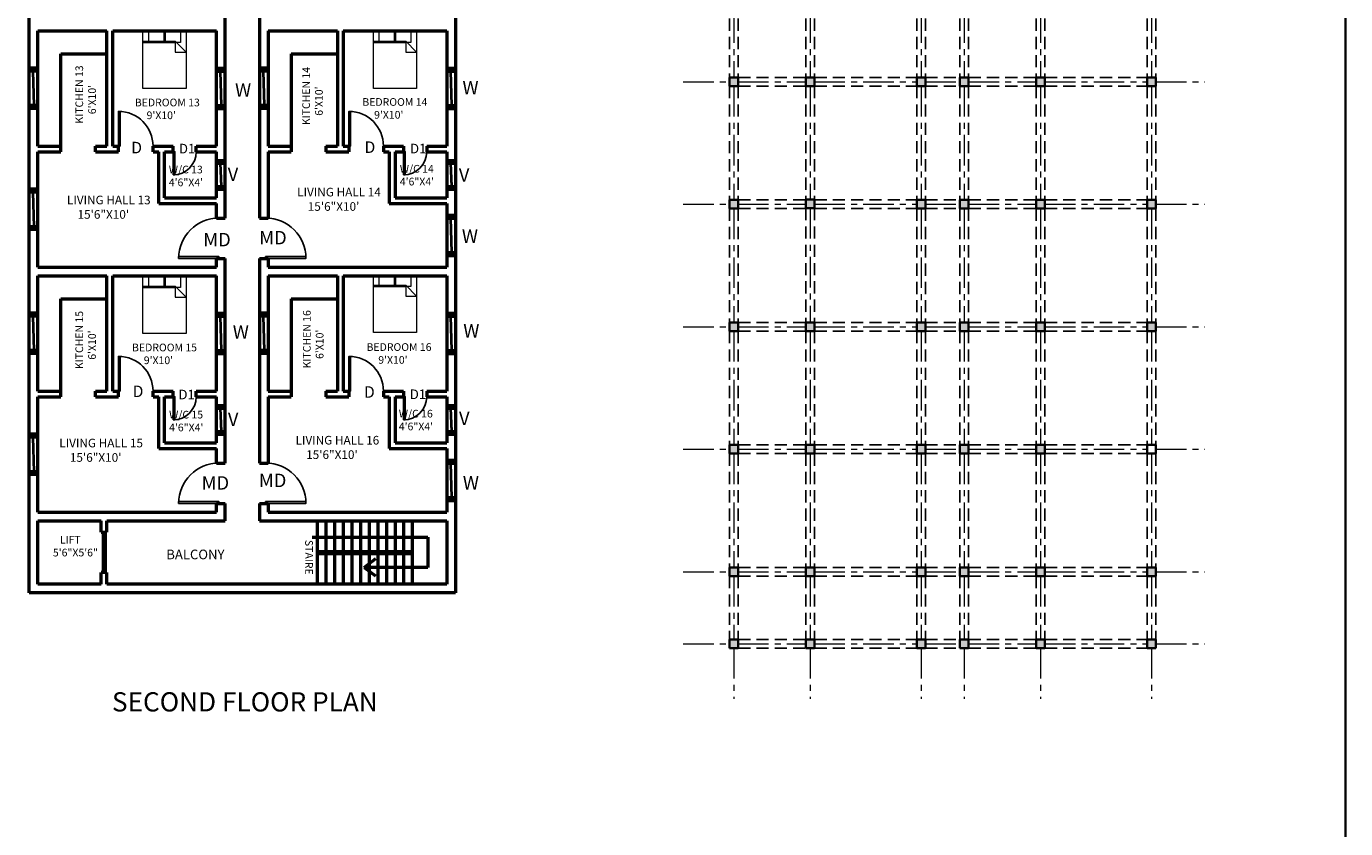
# Model space of a CAD drawing. Units: inches. Extents: x 9239 to 26065, y 6728 to 14611.
# Tile 11 of 12: x 24691 to 26065, y 13102 to 13937. Entities that reach past the tile are written whole.
import ezdxf

# ---------------------------------------------------------------- set-up
doc = ezdxf.new("R2010")
doc.units = ezdxf.units.IN
doc.header["$MEASUREMENT"] = 0
doc.linetypes.add('CENTER', pattern=[50.8, 31.75, -6.35, 6.35, -6.35])
doc.linetypes.add('DASHED', pattern=[19.05, 12.7, -6.35])
for name, color, linetype, lineweight in [('A-ANNO-TEXT', 7, 'Continuous', 18), ('A-ANNO-TTLB', 7, 'Continuous', 35), ('A-AREA-IDEN', 7, 'Continuous', 18), ('A-DOOR', 4, 'Continuous', 25), ('A-FURN', 8, 'Continuous', 18), ('A-GLAZ', 4, 'Continuous', 25), ('A-GRID', 3, 'CENTER', 18), ('A-WALL', 7, 'Continuous', 50), ('S-BEAM', 4, 'DASHED', 25), ('S-COLS', 1, 'Continuous', 35), ('S-PATT', 252, 'Continuous', 13)]:
    doc.layers.add(name, color=color, linetype=linetype, lineweight=lineweight)
doc.styles.get("Standard").update_dxf_attribs({"font": 'arial.ttf'})

# ---------------------------------------------------------------- blocks, each defined once
blk = doc.blocks.new('*U10')
for p, q in [((0, 0), (0, -6)), ((36, 0), (36, -6))]:
    blk.add_line(p, q)
blk.add_lwpolyline([(0, 0), (0, 36), (1.75, 36), (1.75, 0)], close=True)
blk.add_arc((0, 0), 36, 0, 90)
blk = doc.blocks.new('*U34')
for p, q in [((0, 0), (0, 6)), ((24, 0), (24, 6))]:
    blk.add_line(p, q)
blk.add_lwpolyline([(0, 0), (0, -24), (1.75, -24), (1.75, 0)], close=True)
blk.add_arc((0, 0), 24, 270, 0)
blk = doc.blocks.new('*U33')
for p, q in [((-40, 0), (-40, 6)), ((0, 0), (0, 6))]:
    blk.add_line(p, q)
blk.add_lwpolyline([(0, 0), (0, -40), (-1.75, -40), (-1.75, 0)], close=True)
blk.add_arc((0, 0), 40, 180, 270)
blk = doc.blocks.new('*U35')
for p, q in [((0, 0), (0, -6)), ((-40, 0), (-40, -6))]:
    blk.add_line(p, q)
blk.add_lwpolyline([(0, 0), (0, 40), (-1.75, 40), (-1.75, 0)], close=True)
blk.add_arc((0, 0), 40, 90, 180)
blk = doc.blocks.new('Bed - Queen')
for p, q in [((0, -80.00003), (0, 0)), ((0, 0), (59.99999, 0)), ((59.99999, 0), (59.99999, -80.00003)), ((0, -14.4), (44.8, -14.4)), ((44.8, -16.8), (0, -16.8)), ((7.99999, -1.2), (28.79998, -1.2)), ((7.99999, -14.4), (7.99999, -1.2)), ((28.79998, -1.2), (28.79998, -14.4)), ((31.19999, -1.2), (51.99999, -1.2)), ((31.19999, -14.4), (31.19999, -1.2)), ((59.99999, -29.6), (44.8, -14.4)), ((44.8, -14.4), (44.8, -29.6)), ((51.99999, -16.4), (46.79936, -16.4)), ((51.99999, -1.2), (51.99999, -16.4)), ((44.8, -29.6), (59.99999, -29.6)), ((59.99999, -80.00003), (0, -80.00003))]:
    blk.add_line(p, q)
blk = doc.blocks.new('WIN-36')
for p, q in [((0, 1), (36, 1)), ((0, 0.5), (36, 0.5)), ((0, 0), (36, 0))]:
    blk.add_line(p, q)
blk = doc.blocks.new('WIN-24')
for p, q in [((0, 1), (24, 1)), ((0, 0.5), (24, 0.5)), ((0, 0), (24, 0))]:
    blk.add_line(p, q)

msp = doc.modelspace()

# ---------------------------------------------------------------- hatches: boundary and pattern name
at = {"layer": 'S-PATT'}
h = msp.add_hatch(color=256, dxfattribs=at)
h.dxf.hatch_style = 1
h.paths.add_polyline_path([(25432.02, 14384.38), (25432.02, 14393.38), (25423.02, 14393.38), (25423.02, 14384.38)])
h.paths.add_polyline_path([(25511.52, 14384.38), (25511.52, 14393.38), (25502.52, 14393.38), (25502.52, 14384.38)])
h.paths.add_polyline_path([(25627.02, 14384.38), (25627.02, 14393.38), (25618.02, 14393.38), (25618.02, 14384.38)])
h.paths.add_polyline_path([(25672.02, 14393.38), (25663.02, 14393.38), (25663.02, 14384.38), (25672.02, 14384.38)])
h.paths.add_polyline_path([(25742.52, 14384.38), (25751.52, 14384.38), (25751.52, 14393.38), (25742.52, 14393.38)])
h.paths.add_polyline_path([(25858.02, 14384.38), (25867.02, 14384.38), (25867.02, 14393.38), (25858.02, 14393.38)])
h.paths.add_polyline_path([(25423.02, 14256.88), (25432.02, 14256.88), (25432.02, 14265.88), (25423.02, 14265.88)])
h.paths.add_polyline_path([(25502.52, 14256.88), (25511.52, 14256.88), (25511.52, 14265.88), (25502.52, 14265.88)])
h.paths.add_polyline_path([(25618.02, 14256.88), (25627.02, 14256.88), (25627.02, 14265.88), (25618.02, 14265.88)])
h.paths.add_polyline_path([(25672.02, 14265.88), (25663.02, 14265.88), (25663.02, 14256.88), (25672.02, 14256.88)])
h.paths.add_polyline_path([(25751.52, 14256.88), (25751.52, 14265.88), (25742.52, 14265.88), (25742.52, 14256.88)])
h.paths.add_polyline_path([(25858.02, 14256.88), (25867.02, 14256.88), (25867.02, 14265.88), (25858.02, 14265.88)])
h.paths.add_polyline_path([(25423.02, 14129.38), (25432.02, 14129.38), (25432.02, 14138.38), (25423.02, 14138.38)])
h.paths.add_polyline_path([(25511.52, 14129.38), (25511.52, 14138.38), (25502.52, 14138.38), (25502.52, 14129.38)])
h.paths.add_polyline_path([(25618.02, 14129.38), (25627.02, 14129.38), (25627.02, 14138.38), (25618.02, 14138.38)])
h.paths.add_polyline_path([(25672.02, 14138.38), (25663.02, 14138.38), (25663.02, 14129.38), (25672.02, 14129.38)])
h.paths.add_polyline_path([(25742.52, 14129.38), (25751.52, 14129.38), (25751.52, 14138.38), (25742.52, 14138.38)])
h.paths.add_polyline_path([(25867.02, 14129.38), (25867.02, 14138.38), (25858.02, 14138.38), (25858.02, 14129.38)])
h.paths.add_polyline_path([(25432.02, 14010.88), (25423.02, 14010.88), (25423.02, 14001.88), (25432.02, 14001.88)])
h.paths.add_polyline_path([(25502.52, 14010.88), (25502.52, 14001.88), (25511.52, 14001.88), (25511.52, 14010.88)])
h.paths.add_polyline_path([(25618.02, 14001.88), (25627.02, 14001.88), (25627.02, 14010.88), (25618.02, 14010.88)])
h.paths.add_polyline_path([(25672.02, 14001.88), (25672.02, 14010.88), (25663.02, 14010.88), (25663.02, 14001.88)])
h.paths.add_polyline_path([(25751.52, 14010.88), (25742.52, 14010.88), (25742.52, 14001.88), (25751.52, 14001.88)])
h.paths.add_polyline_path([(25867.02, 14010.88), (25858.02, 14010.88), (25858.02, 14001.88), (25867.02, 14001.88)])
h.paths.add_polyline_path([(25432.02, 13874.38), (25432.02, 13883.38), (25423.02, 13883.38), (25423.02, 13874.38)])
h.paths.add_polyline_path([(25502.52, 13874.38), (25511.52, 13874.38), (25511.52, 13883.38), (25502.52, 13883.38)])
h.paths.add_polyline_path([(25627.02, 13883.38), (25618.02, 13883.38), (25618.02, 13874.38), (25627.02, 13874.38)])
h.paths.add_polyline_path([(25672.02, 13874.38), (25672.02, 13883.38), (25663.02, 13883.38), (25663.02, 13874.38)])
h.paths.add_polyline_path([(25751.52, 13883.38), (25742.52, 13883.38), (25742.52, 13874.38), (25751.52, 13874.38)])
h.paths.add_polyline_path([(25858.02, 13874.38), (25867.02, 13874.38), (25867.02, 13883.38), (25858.02, 13883.38)])
h.paths.add_polyline_path([(25432.02, 13746.88), (25432.02, 13755.88), (25423.02, 13755.88), (25423.02, 13746.88)])
h.paths.add_polyline_path([(25502.52, 13747.4), (25511.52, 13747.4), (25511.52, 13756.4), (25502.52, 13756.4)])
h.paths.add_polyline_path([(25627.02, 13746.88), (25627.02, 13755.88), (25618.02, 13755.88), (25618.02, 13746.88)])
h.paths.add_polyline_path([(25672.02, 13746.88), (25672.02, 13755.88), (25663.02, 13755.88), (25663.02, 13746.88)])
h.paths.add_polyline_path([(25742.52, 13746.88), (25751.52, 13746.88), (25751.52, 13755.88), (25742.52, 13755.88)])
h.paths.add_polyline_path([(25867.02, 13746.88), (25867.02, 13755.88), (25858.02, 13755.88), (25858.02, 13746.88)])
h.paths.add_polyline_path([(25423.02, 13619.38), (25432.02, 13619.38), (25432.02, 13628.38), (25423.02, 13628.38)])
h.paths.add_polyline_path([(25511.52, 13619.38), (25511.52, 13628.38), (25502.52, 13628.38), (25502.52, 13619.38)])
h.paths.add_polyline_path([(25627.02, 13619.38), (25627.02, 13628.38), (25618.02, 13628.38), (25618.02, 13619.38)])
h.paths.add_polyline_path([(25672.02, 13619.38), (25672.02, 13628.38), (25663.02, 13628.38), (25663.02, 13619.38)])
h.paths.add_polyline_path([(25751.52, 13628.38), (25742.52, 13628.38), (25742.52, 13619.38), (25751.52, 13619.38)])
h.paths.add_polyline_path([(25858.02, 13619.38), (25867.02, 13619.38), (25867.02, 13628.38), (25858.02, 13628.38)])
h.paths.add_polyline_path([(25423.02, 13491.88), (25432.02, 13491.88), (25432.02, 13500.88), (25423.02, 13500.88)])
h.paths.add_polyline_path([(25511.52, 13500.88), (25502.52, 13500.88), (25502.52, 13491.88), (25511.52, 13491.88)])
h.paths.add_polyline_path([(25627.02, 13491.88), (25627.02, 13500.88), (25618.02, 13500.88), (25618.02, 13491.88)])
h.paths.add_polyline_path([(25663.02, 13491.88), (25672.02, 13491.88), (25672.02, 13500.88), (25663.02, 13500.88)])
h.paths.add_polyline_path([(25742.52, 13491.88), (25751.52, 13491.88), (25751.52, 13500.88), (25742.52, 13500.88)])
h.paths.add_polyline_path([(25432.02, 13373.38), (25423.02, 13373.38), (25423.02, 13364.38), (25432.02, 13364.38)])
h.paths.add_polyline_path([(25502.52, 13373.38), (25502.52, 13364.38), (25511.52, 13364.38), (25511.52, 13373.38)])
h.paths.add_polyline_path([(25618.02, 13373.38), (25618.02, 13364.38), (25627.02, 13364.38), (25627.02, 13373.38)])
h.paths.add_polyline_path([(25663.02, 13373.38), (25663.02, 13364.38), (25672.02, 13364.38), (25672.02, 13373.38)])
h.paths.add_polyline_path([(25742.52, 13373.38), (25742.52, 13364.38), (25751.52, 13364.38), (25751.52, 13373.38)])
h.paths.add_polyline_path([(25858.02, 13373.38), (25858.02, 13364.38), (25867.02, 13364.38), (25867.02, 13373.38)])
h.paths.add_polyline_path([(25432.02, 13298.38), (25423.02, 13298.38), (25423.02, 13289.38), (25432.02, 13289.38)])
h.paths.add_polyline_path([(25511.52, 13298.38), (25502.52, 13298.38), (25502.52, 13289.38), (25511.52, 13289.38)])
h.paths.add_polyline_path([(25618.02, 13298.38), (25618.02, 13289.38), (25627.02, 13289.38), (25627.02, 13298.38)])
h.paths.add_polyline_path([(25663.02, 13298.38), (25663.02, 13289.38), (25672.02, 13289.38), (25672.02, 13298.38)])
h.paths.add_polyline_path([(25742.52, 13298.38), (25742.52, 13289.38), (25751.52, 13289.38), (25751.52, 13298.38)])
h.paths.add_polyline_path([(25858.02, 13298.38), (25858.02, 13289.38), (25867.02, 13289.38), (25867.02, 13298.38)])

# ---------------------------------------------------------------- linework, layer by layer
at = {"layer": 'A-ANNO-TTLB'}
msp.add_lwpolyline([(23324.14, 14611.25), (26064.6, 14611.25), (26064.6, 11591.84), (23324.14, 11591.84)], close=True, dxfattribs=at)
at = {"layer": 'A-GRID'}
for p, q in [((25427.52, 14001.88), (25427.52, 13883.38)), ((25507.02, 14001.88), (25507.02, 13883.38)), ((25622.52, 14001.88), (25622.52, 13883.38)), ((25667.52, 14001.88), (25667.52, 13883.38)), ((25747.02, 14001.88), (25747.02, 13883.38)), ((25862.52, 14001.88), (25862.52, 13883.38)), ((25374.85, 13878.88), (25423.02, 13878.88)), ((25432.02, 13878.88), (25502.52, 13878.88)), ((25511.52, 13878.88), (25618.02, 13878.88)), ((25627.02, 13878.88), (25663.02, 13878.88)), ((25672.02, 13878.88), (25742.52, 13878.88)), ((25751.52, 13878.88), (25858.02, 13878.88)), ((25867.02, 13878.88), (25917.98, 13878.88)), ((25427.52, 13874.38), (25427.52, 13755.88)), ((25507.02, 13874.38), (25507.02, 13756.4)), ((25622.52, 13874.38), (25622.52, 13755.88)), ((25667.52, 13874.38), (25667.52, 13755.88)), ((25747.02, 13874.38), (25747.02, 13755.88)), ((25862.52, 13874.38), (25862.52, 13755.88)), ((25374.85, 13751.38), (25423.02, 13751.38)), ((25427.52, 13746.88), (25427.52, 13628.38)), ((25432.02, 13751.38), (25502.52, 13751.38)), ((25507.02, 13747.4), (25507.02, 13628.38)), ((25511.52, 13751.38), (25618.02, 13751.38)), ((25622.52, 13746.88), (25622.52, 13628.38)), ((25627.02, 13751.38), (25663.02, 13751.38)), ((25667.52, 13746.88), (25667.52, 13628.38)), ((25672.02, 13751.38), (25742.52, 13751.38)), ((25747.02, 13746.88), (25747.02, 13628.38)), ((25751.52, 13751.38), (25858.02, 13751.38)), ((25862.52, 13746.88), (25862.52, 13628.38)), ((25867.02, 13751.38), (25917.98, 13751.38)), ((25374.85, 13623.88), (25423.02, 13623.88)), ((25427.52, 13619.38), (25427.52, 13500.88)), ((25432.02, 13623.88), (25502.52, 13623.88)), ((25507.02, 13619.38), (25507.02, 13500.88)), ((25511.52, 13623.88), (25618.02, 13623.88)), ((25622.52, 13619.38), (25622.52, 13500.88)), ((25627.02, 13623.88), (25663.02, 13623.88)), ((25667.52, 13619.38), (25667.52, 13500.88)), ((25672.02, 13623.88), (25742.52, 13623.88)), ((25747.02, 13619.38), (25747.02, 13500.88)), ((25751.52, 13623.88), (25858.02, 13623.88)), ((25862.52, 13619.38), (25862.52, 13500.88)), ((25867.02, 13623.88), (25917.98, 13623.88)), ((25374.85, 13496.38), (25423.02, 13496.38)), ((25427.52, 13491.88), (25427.52, 13373.38)), ((25432.02, 13496.38), (25502.52, 13496.38)), ((25507.02, 13491.88), (25507.02, 13373.38)), ((25511.52, 13496.38), (25618.02, 13496.38)), ((25622.52, 13491.88), (25622.52, 13373.38)), ((25627.02, 13496.38), (25663.02, 13496.38)), ((25667.52, 13491.88), (25667.52, 13373.38)), ((25672.02, 13496.38), (25742.52, 13496.38)), ((25747.02, 13491.88), (25747.02, 13373.38)), ((25751.52, 13496.38), (25858.02, 13496.38)), ((25862.52, 13491.88), (25862.52, 13373.38)), ((25867.02, 13496.38), (25917.98, 13496.38)), ((25374.85, 13368.88), (25423.02, 13368.88)), ((25432.02, 13368.88), (25502.52, 13368.88)), ((25511.52, 13368.88), (25618.02, 13368.88)), ((25627.02, 13368.88), (25663.02, 13368.88)), ((25672.02, 13368.88), (25742.52, 13368.88)), ((25751.52, 13368.88), (25858.02, 13368.88)), ((25867.02, 13368.88), (25917.98, 13368.88)), ((25427.52, 13364.38), (25427.52, 13298.38)), ((25507.02, 13364.38), (25507.02, 13298.38)), ((25622.52, 13364.38), (25622.52, 13298.38)), ((25667.52, 13364.38), (25667.52, 13298.38)), ((25747.02, 13364.38), (25747.02, 13298.38)), ((25862.52, 13364.38), (25862.52, 13298.38)), ((25374.85, 13293.88), (25423.02, 13293.88)), ((25427.52, 13289.38), (25427.52, 13236.55)), ((25432.02, 13293.88), (25502.52, 13293.88)), ((25507.02, 13289.38), (25507.02, 13236.55)), ((25511.52, 13293.88), (25618.02, 13293.88)), ((25622.52, 13289.38), (25622.52, 13236.55)), ((25627.02, 13293.88), (25663.02, 13293.88)), ((25667.52, 13289.38), (25667.52, 13236.55)), ((25672.02, 13293.88), (25742.52, 13293.88)), ((25747.02, 13289.38), (25747.02, 13236.55)), ((25751.52, 13293.88), (25858.02, 13293.88)), ((25862.52, 13289.38), (25862.52, 13236.55)), ((25867.02, 13293.88), (25917.98, 13293.88))]:
    msp.add_line(p, q, dxfattribs=at)
at = {"layer": 'A-WALL'}
for p, q in [((24693.68, 13347.02), (24693.68, 14451.02)), ((25137.68, 14451.02), (25137.68, 13347.02)), ((24897.68, 13737.02), (24897.68, 13950.02)), ((24933.68, 13950.02), (24933.68, 13737.02)), ((24702.68, 13932.02), (24774.68, 13932.02)), ((24702.68, 13812.02), (24702.68, 13932.02)), ((24774.68, 13812.02), (24774.68, 13932.02)), ((24780.68, 13812.02), (24780.68, 13932.02)), ((24780.68, 13932.02), (24888.68, 13932.02)), ((24888.68, 13812.02), (24888.68, 13932.02)), ((24942.68, 13932.02), (25014.68, 13932.02)), ((24942.68, 13932.02), (24942.68, 13812.02)), ((25014.68, 13932.02), (25014.68, 13812.02)), ((25020.68, 13932.02), (25020.68, 13812.02)), ((25020.68, 13932.02), (25128.68, 13932.02)), ((25128.68, 13932.02), (25128.68, 13812.02)), ((24726.68, 13812.02), (24726.68, 13908.02)), ((24726.68, 13908.02), (24774.68, 13908.02)), ((24966.68, 13908.02), (24966.68, 13812.02)), ((24966.68, 13908.02), (25014.68, 13908.02)), ((24702.68, 13893.02), (24693.68, 13893.02)), ((24702.68, 13890.02), (24693.68, 13890.02)), ((24888.68, 13893.02), (24897.68, 13893.02)), ((24888.68, 13890.02), (24897.68, 13890.02)), ((24942.68, 13893.02), (24933.68, 13893.02)), ((24942.68, 13890.02), (24933.68, 13890.02)), ((25128.68, 13893.02), (25137.68, 13893.02)), ((25128.68, 13890.02), (25137.68, 13890.02)), ((24702.68, 13854.02), (24693.68, 13854.02)), ((24702.68, 13851.02), (24693.68, 13851.02)), ((24888.68, 13854.02), (24897.68, 13854.02)), ((24888.68, 13851.02), (24897.68, 13851.02)), ((24942.68, 13854.02), (24933.68, 13854.02)), ((24942.68, 13851.02), (24933.68, 13851.02)), ((25128.68, 13854.02), (25137.68, 13854.02)), ((25128.68, 13851.02), (25137.68, 13851.02)), ((24702.68, 13812.02), (24726.68, 13812.02)), ((24726.68, 13806.02), (24726.68, 13812.02)), ((24762.68, 13806.02), (24762.68, 13812.02)), ((24762.68, 13812.02), (24774.68, 13812.02)), ((24780.68, 13812.02), (24786.68, 13812.02)), ((24786.68, 13806.02), (24786.68, 13812.02)), ((24822.68, 13806.02), (24822.68, 13812.02)), ((24822.68, 13812.02), (24843.68, 13812.02)), ((24843.68, 13806.02), (24843.68, 13812.02)), ((24867.68, 13806.02), (24867.68, 13812.02)), ((24867.68, 13812.02), (24888.68, 13812.02)), ((24942.68, 13812.02), (24966.68, 13812.02)), ((24966.68, 13812.02), (24966.68, 13806.02)), ((25002.68, 13812.02), (25002.68, 13806.02)), ((25002.68, 13812.02), (25014.68, 13812.02)), ((25020.68, 13812.02), (25026.68, 13812.02)), ((25026.68, 13812.02), (25026.68, 13806.02)), ((25062.68, 13812.02), (25062.68, 13806.02)), ((25062.68, 13812.02), (25083.68, 13812.02)), ((25083.68, 13812.02), (25083.68, 13806.02)), ((25107.68, 13812.02), (25107.68, 13806.02)), ((25107.68, 13812.02), (25128.68, 13812.02)), ((24702.68, 13806.02), (24726.68, 13806.02)), ((24702.68, 13686.02), (24702.68, 13806.02)), ((24762.68, 13806.02), (24786.68, 13806.02)), ((24822.68, 13806.02), (24828.68, 13806.02)), ((24828.68, 13752.02), (24828.68, 13806.02)), ((24834.68, 13758.02), (24834.68, 13806.02)), ((24834.68, 13806.02), (24843.68, 13806.02)), ((24867.68, 13806.02), (24888.68, 13806.02)), ((24888.68, 13758.02), (24888.68, 13806.02)), ((24888.68, 13797.02), (24897.68, 13797.02)), ((24888.68, 13794.02), (24897.68, 13794.02)), ((24942.68, 13806.02), (24966.68, 13806.02)), ((24942.68, 13806.02), (24942.68, 13737.02)), ((25002.68, 13806.02), (25026.68, 13806.02)), ((25062.68, 13806.02), (25068.68, 13806.02)), ((25068.68, 13806.02), (25068.68, 13752.02)), ((25074.68, 13806.02), (25074.68, 13758.02)), ((25074.68, 13806.02), (25083.68, 13806.02)), ((25107.68, 13806.02), (25128.68, 13806.02)), ((25128.68, 13806.02), (25128.68, 13758.02)), ((25128.68, 13797.02), (25137.68, 13797.02)), ((25128.68, 13794.02), (25137.68, 13794.02)), ((24702.68, 13767.02), (24693.68, 13767.02)), ((24888.68, 13770.02), (24897.68, 13770.02)), ((24888.68, 13767.02), (24897.68, 13767.02)), ((25128.68, 13770.02), (25137.68, 13770.02)), ((25128.68, 13767.02), (25137.68, 13767.02)), ((24702.68, 13764.02), (24693.68, 13764.02)), ((24828.68, 13752.02), (24888.68, 13752.02)), ((24834.68, 13758.02), (24888.68, 13758.02)), ((24888.68, 13737.02), (24888.68, 13752.02)), ((25068.68, 13752.02), (25128.68, 13752.02)), ((25074.68, 13758.02), (25128.68, 13758.02)), ((25128.68, 13752.02), (25128.68, 13686.02)), ((25128.68, 13740.02), (25137.68, 13740.02)), ((24702.68, 13728.02), (24693.68, 13728.02)), ((24702.68, 13725.02), (24693.68, 13725.02)), ((24888.68, 13737.02), (24897.68, 13737.02)), ((24933.68, 13737.02), (24942.68, 13737.02)), ((25128.68, 13737.02), (25137.68, 13737.02)), ((25128.68, 13701.02), (25137.68, 13701.02)), ((25128.68, 13698.02), (25137.68, 13698.02)), ((24702.68, 13686.02), (24888.68, 13686.02)), ((24888.68, 13695.02), (24897.68, 13695.02)), ((24888.68, 13686.02), (24888.68, 13695.02)), ((24897.68, 13482.02), (24897.68, 13695.02)), ((24933.68, 13695.02), (24942.68, 13695.02)), ((24933.68, 13695.02), (24933.68, 13482.02)), ((24942.68, 13695.02), (24942.68, 13686.02)), ((24942.68, 13686.02), (25128.68, 13686.02)), ((24702.68, 13677.02), (24774.68, 13677.02)), ((24702.68, 13557.02), (24702.68, 13677.02)), ((24774.68, 13557.02), (24774.68, 13677.02)), ((24780.68, 13557.02), (24780.68, 13677.02)), ((24780.68, 13677.02), (24888.68, 13677.02)), ((24888.68, 13557.02), (24888.68, 13677.02)), ((24942.68, 13677.02), (25014.68, 13677.02)), ((24942.68, 13677.02), (24942.68, 13557.02)), ((25014.68, 13677.02), (25014.68, 13557.02)), ((25020.68, 13677.02), (25020.68, 13557.02)), ((25020.68, 13677.02), (25128.68, 13677.02)), ((25128.68, 13677.02), (25128.68, 13557.02)), ((24726.68, 13557.02), (24726.68, 13653.02)), ((24726.68, 13653.02), (24774.68, 13653.02)), ((24966.68, 13653.02), (24966.68, 13557.02)), ((24966.68, 13653.02), (25014.68, 13653.02)), ((24702.68, 13638.02), (24693.68, 13638.02)), ((24702.68, 13635.02), (24693.68, 13635.02)), ((24888.68, 13638.02), (24897.68, 13638.02)), ((24888.68, 13635.02), (24897.68, 13635.02)), ((24942.68, 13638.02), (24933.68, 13638.02)), ((24942.68, 13635.02), (24933.68, 13635.02)), ((25128.68, 13638.02), (25137.68, 13638.02)), ((25128.68, 13635.02), (25137.68, 13635.02)), ((24702.68, 13599.02), (24693.68, 13599.02)), ((24702.68, 13596.02), (24693.68, 13596.02)), ((24888.68, 13599.02), (24897.68, 13599.02)), ((24888.68, 13596.02), (24897.68, 13596.02)), ((24942.68, 13599.02), (24933.68, 13599.02)), ((24942.68, 13596.02), (24933.68, 13596.02)), ((25128.68, 13599.02), (25137.68, 13599.02)), ((25128.68, 13596.02), (25137.68, 13596.02)), ((24702.68, 13557.02), (24726.68, 13557.02)), ((24702.68, 13551.02), (24726.68, 13551.02)), ((24702.68, 13431.02), (24702.68, 13551.02)), ((24726.68, 13551.02), (24726.68, 13557.02)), ((24762.68, 13551.02), (24762.68, 13557.02)), ((24762.68, 13557.02), (24774.68, 13557.02)), ((24762.68, 13551.02), (24786.68, 13551.02)), ((24780.68, 13557.02), (24786.68, 13557.02)), ((24786.68, 13551.02), (24786.68, 13557.02)), ((24822.68, 13551.02), (24822.68, 13557.02)), ((24822.68, 13557.02), (24843.68, 13557.02)), ((24822.68, 13551.02), (24828.68, 13551.02)), ((24828.68, 13497.02), (24828.68, 13551.02)), ((24834.68, 13503.02), (24834.68, 13551.02)), ((24834.68, 13551.02), (24843.68, 13551.02)), ((24843.68, 13551.02), (24843.68, 13557.02)), ((24867.68, 13551.02), (24867.68, 13557.02)), ((24867.68, 13557.02), (24888.68, 13557.02)), ((24867.68, 13551.02), (24888.68, 13551.02)), ((24888.68, 13503.02), (24888.68, 13551.02)), ((24942.68, 13557.02), (24966.68, 13557.02)), ((24942.68, 13551.02), (24966.68, 13551.02)), ((24942.68, 13551.02), (24942.68, 13482.02)), ((24966.68, 13557.02), (24966.68, 13551.02)), ((25002.68, 13557.02), (25002.68, 13551.02)), ((25002.68, 13557.02), (25014.68, 13557.02)), ((25002.68, 13551.02), (25026.68, 13551.02)), ((25020.68, 13557.02), (25026.68, 13557.02)), ((25026.68, 13557.02), (25026.68, 13551.02)), ((25062.68, 13557.02), (25062.68, 13551.02)), ((25062.68, 13557.02), (25083.68, 13557.02)), ((25062.68, 13551.02), (25068.68, 13551.02)), ((25068.68, 13551.02), (25068.68, 13497.02)), ((25074.68, 13551.02), (25074.68, 13503.02)), ((25074.68, 13551.02), (25083.68, 13551.02)), ((25083.68, 13557.02), (25083.68, 13551.02)), ((25107.68, 13557.02), (25107.68, 13551.02)), ((25107.68, 13557.02), (25128.68, 13557.02)), ((25107.68, 13551.02), (25128.68, 13551.02)), ((25128.68, 13551.02), (25128.68, 13503.02)), ((24888.68, 13542.02), (24897.68, 13542.02)), ((24888.68, 13539.02), (24897.68, 13539.02)), ((25128.68, 13542.02), (25137.68, 13542.02)), ((25128.68, 13539.02), (25137.68, 13539.02)), ((24702.68, 13512.02), (24693.68, 13512.02)), ((24702.68, 13509.02), (24693.68, 13509.02)), ((24888.68, 13515.02), (24897.68, 13515.02)), ((24888.68, 13512.02), (24897.68, 13512.02)), ((25128.68, 13515.02), (25137.68, 13515.02)), ((25128.68, 13512.02), (25137.68, 13512.02)), ((24828.68, 13497.02), (24888.68, 13497.02)), ((24834.68, 13503.02), (24888.68, 13503.02)), ((24888.68, 13482.02), (24888.68, 13497.02)), ((25068.68, 13497.02), (25128.68, 13497.02)), ((25074.68, 13503.02), (25128.68, 13503.02)), ((25128.68, 13497.02), (25128.68, 13431.02)), ((24888.68, 13482.02), (24897.68, 13482.02)), ((24933.68, 13482.02), (24942.68, 13482.02)), ((25128.68, 13485.02), (25137.68, 13485.02)), ((25128.68, 13482.02), (25137.68, 13482.02)), ((24702.68, 13473.02), (24693.68, 13473.02)), ((24702.68, 13470.02), (24693.68, 13470.02)), ((24888.68, 13431.02), (24888.68, 13440.02)), ((24888.68, 13440.02), (24897.68, 13440.02)), ((24897.68, 13422.02), (24897.68, 13440.02)), ((24933.68, 13440.02), (24942.68, 13440.02)), ((24933.68, 13440.02), (24933.68, 13422.02)), ((24942.68, 13440.02), (24942.68, 13431.02)), ((25128.68, 13446.02), (25137.68, 13446.02)), ((25128.68, 13443.02), (25137.68, 13443.02)), ((24702.68, 13431.02), (24888.68, 13431.02)), ((24702.68, 13356.02), (24702.68, 13422.02)), ((24702.68, 13422.02), (24768.68, 13422.02)), ((24768.68, 13410.02), (24768.68, 13422.02)), ((24774.68, 13422.02), (24897.68, 13422.02)), ((24774.68, 13410.02), (24774.68, 13422.02)), ((24933.68, 13422.02), (25128.68, 13422.02)), ((24942.68, 13431.02), (25128.68, 13431.02)), ((24993.68, 13422.02), (24993.68, 13356.02)), ((25002.68, 13422.02), (25002.68, 13390.02)), ((25011.68, 13422.02), (25011.68, 13390.02)), ((25020.68, 13422.02), (25020.68, 13390.02)), ((25029.68, 13422.02), (25029.68, 13390.02)), ((25038.68, 13422.02), (25038.68, 13390.02)), ((25047.68, 13422.02), (25047.68, 13390.02)), ((25056.68, 13422.02), (25056.68, 13390.02)), ((25065.68, 13422.02), (25065.68, 13390.02)), ((25074.68, 13422.02), (25074.68, 13390.02)), ((25083.68, 13422.02), (25083.68, 13390.02)), ((25092.68, 13422.02), (25092.68, 13356.02)), ((25128.68, 13422.02), (25128.68, 13356.02)), ((24768.68, 13410.02), (24774.68, 13410.02)), ((24770.68, 13410.02), (24770.68, 13368.02)), ((24772.68, 13410.02), (24772.68, 13368.02)), ((24988.49, 13404.84), (25108.92, 13404.84)), ((25108.92, 13404.84), (25108.92, 13373.34)), ((24993.68, 13390.02), (25092.68, 13390.02)), ((24993.68, 13388.02), (25092.68, 13388.02)), ((25002.68, 13388.02), (25002.68, 13356.02)), ((25011.68, 13388.02), (25011.68, 13356.02)), ((25020.68, 13388.02), (25020.68, 13356.02)), ((25029.68, 13388.02), (25029.68, 13356.02)), ((25038.68, 13388.02), (25038.68, 13356.02)), ((25042.71, 13373.34), (25054.78, 13382.6)), ((25047.68, 13388.02), (25047.68, 13356.02)), ((25056.68, 13388.02), (25056.68, 13356.02)), ((25065.68, 13388.02), (25065.68, 13356.02)), ((25074.68, 13388.02), (25074.68, 13356.02)), ((25083.68, 13388.02), (25083.68, 13356.02)), ((24768.68, 13356.02), (24768.68, 13368.02)), ((24774.68, 13368.02), (24768.68, 13368.02)), ((24774.68, 13356.02), (24774.68, 13368.02)), ((25108.92, 13373.34), (25042.71, 13373.34)), ((25042.71, 13373.34), (25054.49, 13364.58)), ((24768.68, 13356.02), (24702.68, 13356.02)), ((25128.68, 13356.02), (24774.68, 13356.02)), ((25137.68, 13347.02), (24693.68, 13347.02))]:
    msp.add_line(p, q, dxfattribs=at)
at = {"layer": 'S-BEAM'}
for p, q in [((25423.02, 14001.88), (25423.02, 13883.38)), ((25432.02, 14001.88), (25432.02, 13883.38)), ((25502.52, 14001.88), (25502.52, 13883.38)), ((25511.52, 14001.88), (25511.52, 13883.38)), ((25618.02, 14001.88), (25618.02, 13883.38)), ((25627.02, 14001.88), (25627.02, 13883.38)), ((25663.02, 14001.88), (25663.02, 13883.38)), ((25672.02, 14001.88), (25672.02, 13883.38)), ((25742.52, 14001.88), (25742.52, 13883.38)), ((25751.52, 14001.88), (25751.52, 13883.38)), ((25858.02, 14001.88), (25858.02, 13883.38)), ((25867.02, 14001.88), (25867.02, 13883.38)), ((25432.02, 13883.38), (25502.52, 13883.38)), ((25511.52, 13883.38), (25618.02, 13883.38)), ((25627.02, 13883.38), (25663.02, 13883.38)), ((25672.02, 13883.38), (25742.52, 13883.38)), ((25751.52, 13883.38), (25858.02, 13883.38)), ((25423.02, 13874.38), (25423.02, 13755.88)), ((25432.02, 13874.38), (25502.52, 13874.38)), ((25432.02, 13874.38), (25432.02, 13755.88)), ((25502.52, 13874.38), (25502.52, 13756.4)), ((25511.52, 13874.38), (25618.02, 13874.38)), ((25511.52, 13874.38), (25511.52, 13756.4)), ((25618.02, 13874.38), (25618.02, 13755.88)), ((25627.02, 13874.38), (25663.02, 13874.38)), ((25627.02, 13874.38), (25627.02, 13755.88)), ((25663.02, 13874.38), (25663.02, 13755.88)), ((25672.02, 13874.38), (25742.52, 13874.38)), ((25672.02, 13874.38), (25672.02, 13755.88)), ((25742.52, 13874.38), (25742.52, 13755.88)), ((25751.52, 13874.38), (25858.02, 13874.38)), ((25751.52, 13874.38), (25751.52, 13755.88)), ((25858.02, 13874.38), (25858.02, 13755.88)), ((25867.02, 13874.38), (25867.02, 13755.88)), ((25432.02, 13755.88), (25502.52, 13755.88)), ((25511.52, 13755.88), (25618.02, 13755.88)), ((25627.02, 13755.88), (25663.02, 13755.88)), ((25672.02, 13755.88), (25742.52, 13755.88)), ((25751.52, 13755.88), (25858.02, 13755.88)), ((25423.02, 13746.88), (25423.02, 13628.38)), ((25432.02, 13746.88), (25502.52, 13746.88)), ((25432.02, 13746.88), (25432.02, 13628.38)), ((25502.52, 13747.4), (25502.52, 13628.38)), ((25511.52, 13747.4), (25511.52, 13628.38)), ((25511.52, 13746.88), (25618.02, 13746.88)), ((25618.02, 13746.88), (25618.02, 13628.38)), ((25627.02, 13746.88), (25663.02, 13746.88)), ((25627.02, 13746.88), (25627.02, 13628.38)), ((25663.02, 13746.88), (25663.02, 13628.38)), ((25672.02, 13746.88), (25742.52, 13746.88)), ((25672.02, 13746.88), (25672.02, 13628.38)), ((25742.52, 13746.88), (25742.52, 13628.38)), ((25751.52, 13746.88), (25858.02, 13746.88)), ((25751.52, 13746.88), (25751.52, 13628.38)), ((25858.02, 13746.88), (25858.02, 13628.38)), ((25867.02, 13746.88), (25867.02, 13628.38)), ((25432.02, 13628.38), (25502.52, 13628.38)), ((25511.52, 13628.38), (25618.02, 13628.38)), ((25627.02, 13628.38), (25663.02, 13628.38)), ((25672.02, 13628.38), (25742.52, 13628.38)), ((25751.52, 13628.38), (25858.02, 13628.38)), ((25423.02, 13619.38), (25423.02, 13500.88)), ((25432.02, 13619.38), (25502.52, 13619.38)), ((25432.02, 13619.38), (25432.02, 13500.88)), ((25502.52, 13619.38), (25502.52, 13500.88)), ((25511.52, 13619.38), (25618.02, 13619.38)), ((25511.52, 13619.38), (25511.52, 13500.88)), ((25618.02, 13619.38), (25618.02, 13500.88)), ((25627.02, 13619.38), (25663.02, 13619.38)), ((25627.02, 13619.38), (25627.02, 13500.88)), ((25663.02, 13619.38), (25663.02, 13500.88)), ((25672.02, 13619.38), (25742.52, 13619.38)), ((25672.02, 13619.38), (25672.02, 13500.88)), ((25742.52, 13619.38), (25742.52, 13500.88)), ((25751.52, 13619.38), (25858.02, 13619.38)), ((25751.52, 13619.38), (25751.52, 13500.88)), ((25858.02, 13619.38), (25858.02, 13500.88)), ((25867.02, 13619.38), (25867.02, 13500.88)), ((25423.02, 13491.88), (25423.02, 13373.38)), ((25432.02, 13500.88), (25502.52, 13500.88)), ((25432.02, 13491.88), (25502.52, 13491.88)), ((25432.02, 13491.88), (25432.02, 13373.38)), ((25502.52, 13491.88), (25502.52, 13373.38)), ((25511.52, 13500.88), (25618.02, 13500.88)), ((25511.52, 13491.88), (25618.02, 13491.88)), ((25511.52, 13491.88), (25511.52, 13373.38)), ((25618.02, 13491.88), (25618.02, 13373.38)), ((25627.02, 13500.88), (25663.02, 13500.88)), ((25627.02, 13491.88), (25663.02, 13491.88)), ((25627.02, 13491.88), (25627.02, 13373.38)), ((25663.02, 13491.88), (25663.02, 13373.38)), ((25672.02, 13500.88), (25742.52, 13500.88)), ((25672.02, 13491.88), (25742.52, 13491.88)), ((25672.02, 13491.88), (25672.02, 13373.38)), ((25742.52, 13491.88), (25742.52, 13373.38)), ((25751.52, 13500.88), (25858.02, 13500.88)), ((25751.52, 13491.88), (25858.02, 13491.88)), ((25751.52, 13491.88), (25751.52, 13373.38)), ((25858.02, 13491.88), (25858.02, 13373.38)), ((25867.02, 13491.88), (25867.02, 13373.38)), ((25432.02, 13373.38), (25502.52, 13373.38)), ((25511.52, 13373.38), (25618.02, 13373.38)), ((25627.02, 13373.38), (25663.02, 13373.38)), ((25672.02, 13373.38), (25742.52, 13373.38)), ((25751.52, 13373.38), (25858.02, 13373.38)), ((25423.02, 13364.38), (25423.02, 13298.38)), ((25432.02, 13364.38), (25502.52, 13364.38)), ((25432.02, 13364.38), (25432.02, 13298.38)), ((25502.52, 13364.38), (25502.52, 13298.38)), ((25511.52, 13364.38), (25618.02, 13364.38)), ((25511.52, 13364.38), (25511.52, 13298.38)), ((25618.02, 13364.38), (25618.02, 13298.38)), ((25627.02, 13364.38), (25663.02, 13364.38)), ((25627.02, 13364.38), (25627.02, 13298.38)), ((25663.02, 13364.38), (25663.02, 13298.38)), ((25672.02, 13364.38), (25742.52, 13364.38)), ((25672.02, 13364.38), (25672.02, 13298.38)), ((25742.52, 13364.38), (25742.52, 13298.38)), ((25751.52, 13364.38), (25858.02, 13364.38)), ((25751.52, 13364.38), (25751.52, 13298.38)), ((25858.02, 13364.38), (25858.02, 13298.38)), ((25867.02, 13364.38), (25867.02, 13298.38)), ((25432.02, 13298.38), (25502.52, 13298.38)), ((25511.52, 13298.38), (25618.02, 13298.38)), ((25627.02, 13298.38), (25663.02, 13298.38)), ((25672.02, 13298.38), (25742.52, 13298.38)), ((25751.52, 13298.38), (25858.02, 13298.38)), ((25432.02, 13289.38), (25502.52, 13289.38)), ((25511.52, 13289.38), (25618.02, 13289.38)), ((25627.02, 13289.38), (25663.02, 13289.38)), ((25672.02, 13289.38), (25742.52, 13289.38)), ((25751.52, 13289.38), (25858.02, 13289.38))]:
    msp.add_line(p, q, dxfattribs=at)
at = {"layer": 'S-COLS'}
for p, q in [((25423.02, 13883.38), (25432.02, 13883.38)), ((25423.02, 13874.38), (25423.02, 13883.38)), ((25432.02, 13874.38), (25432.02, 13883.38)), ((25432.02, 13883.38), (25432.02, 13874.38)), ((25502.52, 13883.38), (25511.52, 13883.38)), ((25502.52, 13874.38), (25502.52, 13883.38)), ((25511.52, 13883.38), (25511.52, 13874.38)), ((25618.02, 13883.38), (25627.02, 13883.38)), ((25618.02, 13874.38), (25618.02, 13883.38)), ((25627.02, 13883.38), (25627.02, 13874.38)), ((25663.02, 13883.38), (25672.02, 13883.38)), ((25663.02, 13874.38), (25663.02, 13883.38)), ((25672.02, 13883.38), (25672.02, 13874.38)), ((25742.52, 13883.38), (25751.52, 13883.38)), ((25742.52, 13874.38), (25742.52, 13883.38)), ((25751.52, 13883.38), (25751.52, 13874.38)), ((25858.02, 13883.38), (25867.02, 13883.38)), ((25858.02, 13874.38), (25858.02, 13883.38)), ((25867.02, 13883.38), (25867.02, 13874.38)), ((25432.02, 13874.38), (25423.02, 13874.38)), ((25511.52, 13874.38), (25502.52, 13874.38)), ((25627.02, 13874.38), (25618.02, 13874.38)), ((25672.02, 13874.38), (25663.02, 13874.38)), ((25751.52, 13874.38), (25742.52, 13874.38)), ((25867.02, 13874.38), (25858.02, 13874.38)), ((25423.02, 13755.88), (25432.02, 13755.88)), ((25423.02, 13746.88), (25423.02, 13755.88)), ((25432.02, 13755.88), (25432.02, 13746.88)), ((25432.02, 13748.38), (25432.02, 13754.38)), ((25502.52, 13756.4), (25511.52, 13756.4)), ((25502.52, 13747.4), (25502.52, 13756.4)), ((25511.52, 13756.4), (25511.52, 13747.4)), ((25618.02, 13755.88), (25627.02, 13755.88)), ((25618.02, 13746.88), (25618.02, 13755.88)), ((25627.02, 13755.88), (25627.02, 13746.88)), ((25663.02, 13755.88), (25672.02, 13755.88)), ((25663.02, 13746.88), (25663.02, 13755.88)), ((25672.02, 13755.88), (25672.02, 13746.88)), ((25742.52, 13755.88), (25751.52, 13755.88)), ((25742.52, 13746.88), (25742.52, 13755.88)), ((25751.52, 13755.88), (25751.52, 13746.88)), ((25858.02, 13755.88), (25867.02, 13755.88)), ((25858.02, 13746.88), (25858.02, 13755.88)), ((25867.02, 13755.88), (25867.02, 13746.88)), ((25432.02, 13746.88), (25423.02, 13746.88)), ((25511.52, 13747.4), (25502.52, 13747.4)), ((25627.02, 13746.88), (25618.02, 13746.88)), ((25672.02, 13746.88), (25663.02, 13746.88)), ((25751.52, 13746.88), (25742.52, 13746.88)), ((25867.02, 13746.88), (25858.02, 13746.88)), ((25423.02, 13628.38), (25432.02, 13628.38)), ((25423.02, 13619.38), (25423.02, 13628.38)), ((25432.02, 13619.38), (25432.02, 13628.38)), ((25432.02, 13628.38), (25432.02, 13619.38)), ((25502.52, 13628.38), (25511.52, 13628.38)), ((25502.52, 13619.38), (25502.52, 13628.38)), ((25511.52, 13628.38), (25511.52, 13619.38)), ((25618.02, 13628.38), (25627.02, 13628.38)), ((25618.02, 13619.38), (25618.02, 13628.38)), ((25627.02, 13628.38), (25627.02, 13619.38)), ((25663.02, 13628.38), (25672.02, 13628.38)), ((25663.02, 13619.38), (25663.02, 13628.38)), ((25672.02, 13628.38), (25672.02, 13619.38)), ((25742.52, 13628.38), (25751.52, 13628.38)), ((25742.52, 13619.38), (25742.52, 13628.38)), ((25751.52, 13628.38), (25751.52, 13619.38)), ((25858.02, 13628.38), (25867.02, 13628.38)), ((25858.02, 13619.38), (25858.02, 13628.38)), ((25867.02, 13628.38), (25867.02, 13619.38)), ((25432.02, 13619.38), (25423.02, 13619.38)), ((25511.52, 13619.38), (25502.52, 13619.38)), ((25627.02, 13619.38), (25618.02, 13619.38)), ((25672.02, 13619.38), (25663.02, 13619.38)), ((25751.52, 13619.38), (25742.52, 13619.38)), ((25867.02, 13619.38), (25858.02, 13619.38)), ((25423.02, 13500.88), (25432.02, 13500.88)), ((25423.02, 13491.88), (25423.02, 13500.88)), ((25432.02, 13491.88), (25423.02, 13491.88)), ((25432.02, 13500.88), (25432.02, 13491.88)), ((25432.02, 13493.38), (25432.02, 13499.38)), ((25502.52, 13500.88), (25511.52, 13500.88)), ((25502.52, 13491.88), (25502.52, 13500.88)), ((25511.52, 13491.88), (25502.52, 13491.88)), ((25511.52, 13500.88), (25511.52, 13491.88)), ((25618.02, 13500.88), (25627.02, 13500.88)), ((25618.02, 13491.88), (25618.02, 13500.88)), ((25627.02, 13491.88), (25618.02, 13491.88)), ((25627.02, 13500.88), (25627.02, 13491.88)), ((25663.02, 13500.88), (25672.02, 13500.88)), ((25663.02, 13491.88), (25663.02, 13500.88)), ((25672.02, 13491.88), (25663.02, 13491.88)), ((25672.02, 13500.88), (25672.02, 13491.88)), ((25742.52, 13500.88), (25751.52, 13500.88)), ((25742.52, 13491.88), (25742.52, 13500.88)), ((25751.52, 13491.88), (25742.52, 13491.88)), ((25751.52, 13500.88), (25751.52, 13491.88)), ((25858.02, 13500.88), (25867.02, 13500.88)), ((25858.02, 13491.88), (25858.02, 13500.88)), ((25867.02, 13491.88), (25858.02, 13491.88)), ((25867.02, 13500.88), (25867.02, 13491.88)), ((25423.02, 13373.38), (25432.02, 13373.38)), ((25423.02, 13364.38), (25423.02, 13373.38)), ((25432.02, 13364.38), (25432.02, 13373.38)), ((25432.02, 13373.38), (25432.02, 13364.38)), ((25502.52, 13373.38), (25511.52, 13373.38)), ((25502.52, 13364.38), (25502.52, 13373.38)), ((25511.52, 13373.38), (25511.52, 13364.38)), ((25618.02, 13373.38), (25627.02, 13373.38)), ((25618.02, 13364.38), (25618.02, 13373.38)), ((25627.02, 13373.38), (25627.02, 13364.38)), ((25663.02, 13373.38), (25672.02, 13373.38)), ((25663.02, 13364.38), (25663.02, 13373.38)), ((25672.02, 13373.38), (25672.02, 13364.38)), ((25742.52, 13373.38), (25751.52, 13373.38)), ((25742.52, 13364.38), (25742.52, 13373.38)), ((25751.52, 13373.38), (25751.52, 13364.38)), ((25858.02, 13373.38), (25867.02, 13373.38)), ((25858.02, 13364.38), (25858.02, 13373.38)), ((25867.02, 13373.38), (25867.02, 13364.38)), ((25432.02, 13364.38), (25423.02, 13364.38)), ((25511.52, 13364.38), (25502.52, 13364.38)), ((25627.02, 13364.38), (25618.02, 13364.38)), ((25672.02, 13364.38), (25663.02, 13364.38)), ((25751.52, 13364.38), (25742.52, 13364.38)), ((25867.02, 13364.38), (25858.02, 13364.38)), ((25423.02, 13298.38), (25432.02, 13298.38)), ((25423.02, 13289.38), (25423.02, 13298.38)), ((25432.02, 13298.38), (25432.02, 13289.38)), ((25432.02, 13298.38), (25432.02, 13289.38)), ((25502.52, 13298.38), (25511.52, 13298.38)), ((25502.52, 13289.38), (25502.52, 13298.38)), ((25511.52, 13298.38), (25511.52, 13289.38)), ((25618.02, 13298.38), (25627.02, 13298.38)), ((25618.02, 13289.38), (25618.02, 13298.38)), ((25627.02, 13298.38), (25627.02, 13289.38)), ((25663.02, 13298.38), (25672.02, 13298.38)), ((25663.02, 13289.38), (25663.02, 13298.38)), ((25672.02, 13298.38), (25672.02, 13289.38)), ((25742.52, 13298.38), (25751.52, 13298.38)), ((25742.52, 13289.38), (25742.52, 13298.38)), ((25751.52, 13298.38), (25751.52, 13289.38)), ((25858.02, 13298.38), (25867.02, 13298.38)), ((25858.02, 13289.38), (25858.02, 13298.38)), ((25867.02, 13298.38), (25867.02, 13289.38)), ((25432.02, 13289.38), (25423.02, 13289.38)), ((25511.52, 13289.38), (25502.52, 13289.38)), ((25627.02, 13289.38), (25618.02, 13289.38)), ((25672.02, 13289.38), (25663.02, 13289.38)), ((25751.52, 13289.38), (25742.52, 13289.38)), ((25867.02, 13289.38), (25858.02, 13289.38))]:
    msp.add_line(p, q, dxfattribs=at)

# ---------------------------------------------------------------- block references
at = {"layer": 'A-DOOR'}
for name, p in [('*U10', (24786.68, 13812.02)), ('*U10', (25026.68, 13812.02)), ('*U34', (24843.68, 13806.02)), ('*U34', (25083.68, 13806.02)), ('*U10', (24786.68, 13557.02)), ('*U10', (25026.68, 13557.02)), ('*U34', (24843.68, 13551.02)), ('*U34', (25083.68, 13551.02))]:
    msp.add_blockref(name, p, dxfattribs=at)
at = {"layer": 'A-DOOR', "rotation": 270}
for name, p, xscale, yscale, zscale in [('*U33', (24891.38, 13695.02), 1.050000000000002, 1.050000000000002, 1.050000000000002), ('*U35', (24939.98, 13695.02), 1.05, 1.05, 1.05), ('*U33', (24891.38, 13440.02), 1.05, 1.05, 1.05), ('*U35', (24939.98, 13440.02), 1.05, 1.05, 1.05)]:
    msp.add_blockref(name, p, dxfattribs=dict(at, xscale=xscale, yscale=yscale, zscale=zscale))
at = {"layer": 'A-FURN', "xscale": 0.75, "yscale": 0.75, "zscale": 0.75}
for p in [(24812.18, 13932.02), (25052.18, 13932.02), (24812.18, 13677.02), (25052.18, 13677.99)]:
    msp.add_blockref('Bed - Queen', p, dxfattribs=at)
at = {"layer": 'A-GLAZ'}
for name, p, rotation in [('WIN-36', (24697.18, 13890), 271.5911402712003), ('WIN-36', (24892.18, 13890), 271.5911402712003), ('WIN-36', (24937.18, 13890), 271.5911402712003), ('WIN-36', (25132.18, 13890), 271.5911402712235), ('WIN-24', (24892.18, 13793.99), 272.3859440303975), ('WIN-24', (25132.18, 13793.99), 272.3859440304322), ('WIN-36', (24697.18, 13764), 271.5911402712003), ('WIN-36', (25132.18, 13737), 271.5911402712003), ('WIN-36', (24697.18, 13635), 271.5911402712003), ('WIN-36', (24892.18, 13635), 271.5911402712003), ('WIN-36', (24937.18, 13635), 271.5911402712003), ('WIN-36', (25132.18, 13635), 271.5911402712003), ('WIN-24', (24892.18, 13538.99), 272.3859440303975), ('WIN-24', (25132.18, 13538.99), 272.3859440303975), ('WIN-36', (24697.18, 13509), 271.5911402712003), ('WIN-36', (25132.18, 13482), 271.5911402712003)]:
    msp.add_blockref(name, p, dxfattribs=dict(at, rotation=rotation))

# ---------------------------------------------------------------- texts
at = {"layer": 'A-ANNO-TEXT', "attachment_point": 1}
for s, width, insert, char_height in [('W', 545.3335, (24908.08, 13877.36), 14), ('W', 545.3335, (25144.91, 13879.83), 14), ('D', 545.3335, (24799.99, 13816.37), 12), ('D1', 545.3335, (24849.71, 13814.31), 10), ('D', 545.3335, (25042.92, 13816.82), 12), ('D1', 545.3335, (25090.38, 13814.37), 10), ('W/C 14\\P4\'6"X4\'', 1026.6179, (25079.69, 13792.3), 8), ('W/C 13\\P4\'6"X4\'', 1026.6179, (24839.12, 13791.51), 8), ('V', 545.3335, (24900.45, 13789.62), 14), ('V', 545.3335, (25141.13, 13788.9), 14), ('W', 545.3335, (25144.32, 13725.24), 14), ('MD', 545.3335, (24875.01, 13721.57), 14), ('MD', 545.3335, (24933.27, 13723.61), 14), ('W', 545.3335, (24905.73, 13625.47), 14), ('W', 545.3335, (25145.79, 13626.65), 14), ('D', 545.3335, (24801.43, 13562.67), 12), ('D', 545.3335, (25042.34, 13561.98), 12), ('D1', 545.3335, (24849.22, 13558.34), 10), ('D1', 545.3335, (25090.12, 13558.61), 10), ('W/C 15\\P4\'6"X4\'', 1026.6179, (24839.44, 13536.41), 8), ('V', 545.3335, (24900.64, 13534.61), 14), ('W/C 16\\P4\'6"X4\'', 1026.6179, (25078.64, 13537.44), 8), ('V', 545.3335, (25141.33, 13535.52), 14), ('MD', 545.3335, (24873.31, 13468.36), 14), ('MD', 545.3335, (24932.91, 13470.95), 14), ('W', 545.3335, (25145.34, 13468.46), 14), ('   LIFT\\P5\'6"X5\'6"', 441.5638, (24718.43, 13406.18), 8), ('SECOND FLOOR PLAN', 1203.1671, (24779.92, 13243.48), 20)]:
    msp.add_mtext_dynamic_manual_height_columns(s, width=width, gutter_width=1, heights=[0], dxfattribs=dict(at, insert=insert, char_height=char_height))
at = {"layer": 'A-AREA-IDEN', "char_height": 8, "attachment_point": 1}
for s, width, insert, rotation in [("KITCHEN 13\\P    6'X10'", 757.9977, (24741.89, 13835.33), 90), ("KITCHEN 14\\P    6'X10'", 757.9977, (24978.12, 13833.72), 90), ("KITCHEN 15\\P    6'X10'", 757.9977, (24741.85, 13579.8), 90), ("KITCHEN 16\\P    6'X10'", 757.9977, (24978.88, 13580.61), 90), ('STAIRE', 294.5156, (24989.14, 13402.06), 270)]:
    msp.add_mtext_dynamic_manual_height_columns(s, width=width, gutter_width=1, heights=[0], dxfattribs=dict(at, insert=insert, rotation=rotation))
at = {"layer": 'A-AREA-IDEN', "attachment_point": 1}
for s, width, insert, char_height in [("BEDROOM 14\\P     9'X10'", 562.7126, (25040.7, 13861.84), 8), ("BEDROOM 13\\P     9'X10'", 562.7126, (24803.77, 13861.32), 8), ('LIVING HALL 14\\P    15\'6"X10\'', 436.6568, (24972.81, 13768.56), 9), ('LIVING HALL 13\\P    15\'6"X10\'', 436.6568, (24733.06, 13760.33), 9), ("BEDROOM 15\\P     9'X10'", 562.7126, (24800.85, 13606.31), 8), ("BEDROOM 16\\P     9'X10'", 562.7126, (25045.04, 13606.75), 8), ('LIVING HALL 15\\P    15\'6"X10\'', 436.6568, (24725.08, 13507.35), 9), ('LIVING HALL 16\\P    15\'6"X10\'', 436.6568, (24971.13, 13510.3), 9), ('BALCONY', 294.5156, (24836.5, 13391.91), 10)]:
    msp.add_mtext_dynamic_manual_height_columns(s, width=width, gutter_width=1, heights=[0], dxfattribs=dict(at, insert=insert, char_height=char_height))

doc.saveas('drawing.dxf')
